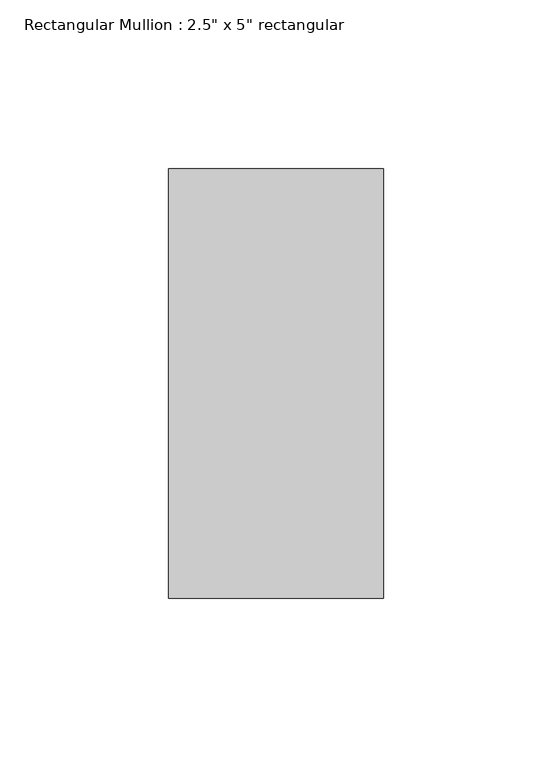
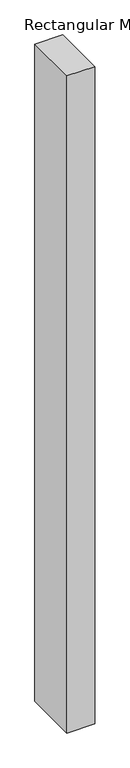
"""IFC4 building model written with IfcOpenShell, lengths in millimetres: member geometry."""

from ifc_helpers import new_model, si_unit, frame, origin, place, context, project, spatial, polyline, outline, extrude, source, transform, mapped, element, save


def member_18747f1d(model_context):
    return source(origin(), model_context, "Body", "SweptSolid", [
        extrude(outline(polyline([(0.0, 63.5), (0.0, -63.5), (-63.5, -63.5), (-63.5, 63.5), (0.0, 63.5)])), frame((0.0, 0.0, -1589.6963029), z_axis=(0.0, 0.0, 1.0), x_axis=(1.0, 0.0, 0.0)), (0.0, 0.0, 1.0), 1589.6963029),
    ])


if __name__ == "__main__":
    model = new_model("IFC4")
    model_context = context("Model", 3, world=origin())
    ifc_project = project(units=[si_unit("LENGTHUNIT", "METRE", prefix="MILLI")], contexts=[model_context])
    site = spatial("IfcSite", under=ifc_project)
    building = spatial("IfcBuilding", under=site)
    placement = place(None, origin())
    member_shape = member_18747f1d(model_context)
    element("IfcMember", 1, ObjectType="Rectangular Mullion : 2.5\" x 5\" rectangular", at=placement, inside=building, context=model_context, shape_type="MappedRepresentation", body=[
        mapped(member_shape, transform((0.0, 0.0, 0.0), x_axis=(1.0, 0.0, 0.0), y_axis=(0.0, 1.0, 0.0), z_axis=(0.0, 0.0, 1.0))),
    ])
    save(model, "model.ifc")

# Revit data of these elements
# Type "Rectangular Mullion : 2.5\" x 5\" rectangular"
#   built-in parameter 1007304 = 0.416667 (stored number, unit not read)
#   built-in parameter 1007301 = 0.104167 (stored number, unit not read)
#   built-in parameter 1007300 = 0.104167 (stored number, unit not read)
# Element 1 (IfcMember, "Rectangular Mullion : 2.5\" x 5\" rectangular")
#   Materials on its faces: "Aluminum"
# Materials
#   "Aluminum": class "Metal", colour RGB 247 247 247, transparency 0, Description = "Aluminum 6061", Cost = 0
